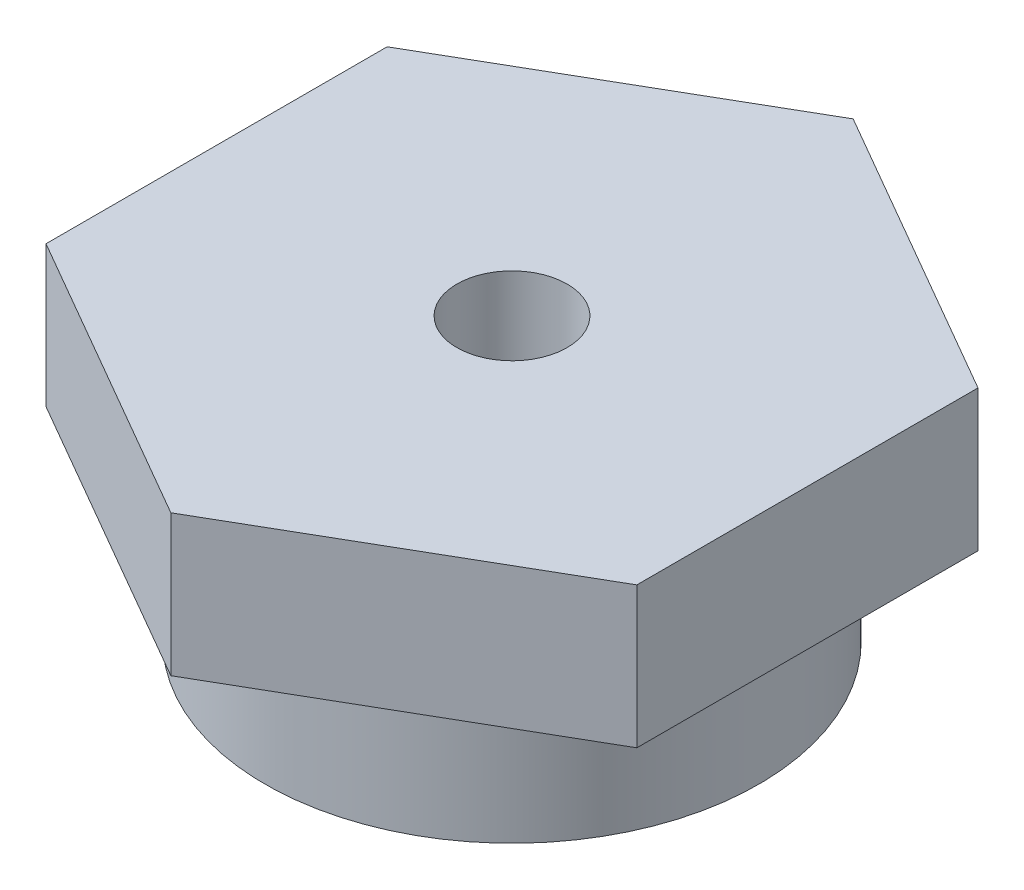
from build123d import *

# Parameters (mm, degrees)
HEX_BODY_67AF_X16_DEPTH = 16
COLLAR_PROFILE_56_R     = 28
COLLAR_56_X16_DEPTH     = 16
BORE_PROFILE_12_5_R     = 6.25
BORE_12_5_THROUGH_DEPTH = 61.353817885


with BuildPart() as part:
    # Hex Profile 67AF → Hex Body 67AF x16 (new body)
    with BuildSketch(Plane(origin=(0, 0, 0), x_dir=(1, 0, 0), z_dir=(0, 1, 0))):
        Polygon((0, -38.682468036), (33.5, -19.341234018), (33.5, 19.341234018), (0, 38.682468036), (-33.5, 19.341234018), (-33.5, -19.341234018), align=None)
    extrude(amount=HEX_BODY_67AF_X16_DEPTH)

    # Collar Profile Ø56 → Collar Ø56 x16 (add)
    with BuildSketch(Plane.XZ):
        with Locations(Location((0, 0, 0), (0, 0, 270))):
            Circle(COLLAR_PROFILE_56_R)
    extrude(amount=COLLAR_56_X16_DEPTH)

    # Bore Profile Ø12.5 → Bore Ø12.5 Through (cut, through all)
    with BuildSketch(Plane.XZ.offset(16)):
        with Locations(Location((0, 0, 0), (0, 0, 270))):
            Circle(BORE_PROFILE_12_5_R)
    extrude(amount=-BORE_12_5_THROUGH_DEPTH, mode=Mode.SUBTRACT)


solid = part.part
